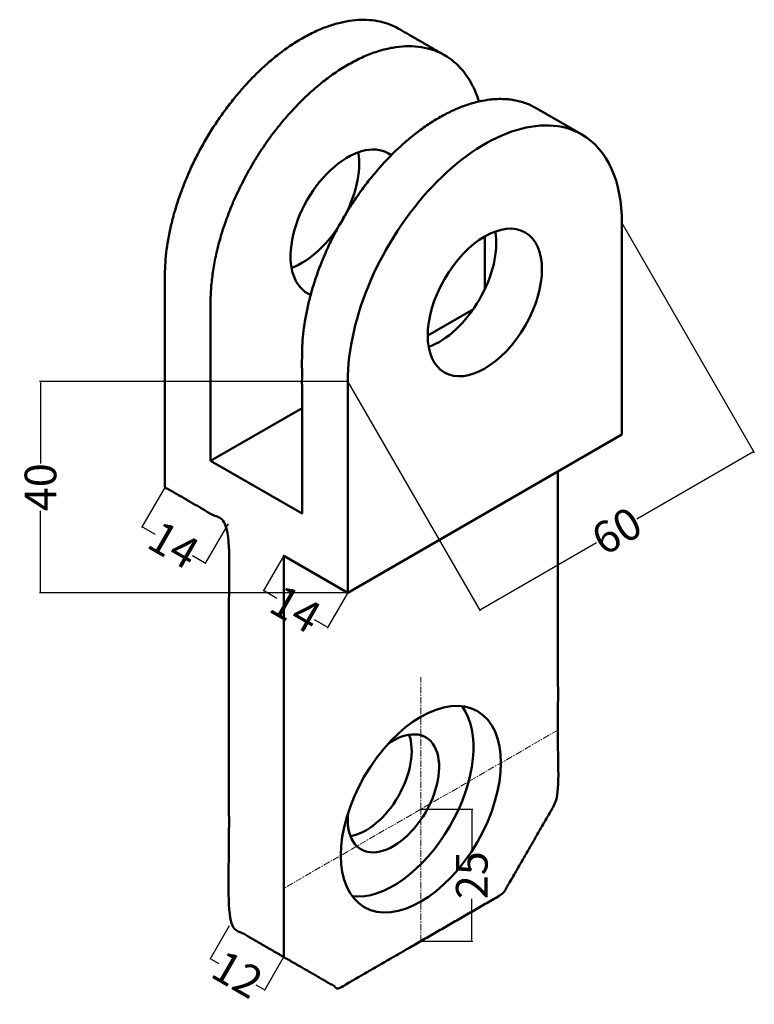
# Model space of a CAD drawing. Units: millimetres. Extents: x 4 to 143, y 22 to 208.
import ezdxf

# ---------------------------------------------------------------- set-up
doc = ezdxf.new("R2010")
doc.units = ezdxf.units.MM
doc.header["$MEASUREMENT"] = 0
doc.linetypes.add('CENTER', pattern=[2, 1.25, -0.25, 0.25, -0.25])
for name, color, linetype, lineweight in [('M-CNTR', 1, 'CENTER', 18), ('M-DIMS', 2, 'Continuous', 25), ('M-OUTL', 7, 'Continuous', 50)]:
    doc.layers.add(name, color=color, linetype=linetype, lineweight=lineweight)
doc.styles.get("Standard").update_dxf_attribs({"font": 'arial.ttf'})
doc.dimstyles.get("Standard").update_dxf_attribs({"dimtxt": 6, "dimasz": 0.18, "dimexe": 0.18, "dimexo": 0.0625, "dimgap": 0.09, "dimtad": 0, "dimtoh": 1, "dimdec": 0, "dimzin": 0, "dimdsep": 46, "dimtxsty": 'Standard', "dimcen": 0.09, "dimadec": 0, "dimazin": 0, "dimtfac": 1, "dimtdec": 0, "dimtofl": 0, "dimtmove": 0, "dimatfit": 3, "dimfxl": 1, "dimtolj": 1, "dimtzin": 0, "dimarcsym": 0})

# ---------------------------------------------------------------- blocks, each defined once
blk = doc.blocks.new('*D1')
at = {"layer": 'Defpoints', "color": 0, "transparency": 16777216}
for p in [(53.96, 106.73), (66.08, 99.73), (62.29, 93.16)]:
    blk.add_point(p, dxfattribs=at)
at = {"layer": 'M-DIMS', "color": 0, "lineweight": -2, "transparency": 16777216}
for p, q in [((53.93, 106.68), (50.07, 100.01)), ((50.32, 100.07), (52.68, 98.71)), ((66.05, 99.68), (62.2, 93.01)), ((62.13, 93.25), (59.77, 94.62))]:
    blk.add_line(p, q, dxfattribs=at)
at = {"layer": 'M-DIMS', "color": 0, "transparency": 16777216}
for points in [[(50.33, 100.1), (50.3, 100.05), (50.16, 100.16)], [(62.15, 93.28), (62.12, 93.23), (62.29, 93.16)]]:
    blk.add_solid(points, dxfattribs=at)
at = {"layer": 'M-DIMS', "color": 0, "transparency": 16777216, "insert": (56.23, 96.66), "char_height": 6, "attachment_point": 5, "rotation": 330}
blk.add_mtext('\\A1;14', dxfattribs=at)
blk = doc.blocks.new('*D2')
at = {"layer": 'Defpoints', "color": 0, "transparency": 16777216}
for p in [(31.44, 119.73), (27.12, 112.26), (43.43, 112.81)]:
    blk.add_point(p, dxfattribs=at)
at = {"layer": 'M-DIMS', "color": 0, "lineweight": -2, "transparency": 16777216}
for p, q in [((31.41, 119.68), (27.03, 112.1)), ((27.28, 112.17), (29.58, 110.84)), ((43.4, 112.76), (39.03, 105.18)), ((38.96, 105.42), (36.67, 106.75))]:
    blk.add_line(p, q, dxfattribs=at)
at = {"layer": 'M-DIMS', "color": 0, "transparency": 16777216}
for points in [[(27.3, 112.19), (27.27, 112.14), (27.12, 112.26)], [(38.98, 105.45), (38.95, 105.4), (39.12, 105.33)]]:
    blk.add_solid(points, dxfattribs=at)
at = {"layer": 'M-DIMS', "color": 0, "transparency": 16777216, "insert": (33.12, 108.79), "char_height": 6, "attachment_point": 5, "rotation": 330}
blk.add_mtext('\\A1;14', dxfattribs=at)
blk = doc.blocks.new('*D3')
at = {"layer": 'Defpoints', "color": 0, "transparency": 16777216}
for p in [(43.66, 36.68), (40.05, 30.42), (53.96, 30.73)]:
    blk.add_point(p, dxfattribs=at)
at = {"layer": 'M-DIMS', "color": 0, "lineweight": -2, "transparency": 16777216}
for p, q in [((43.63, 36.62), (39.96, 30.26)), ((40.21, 30.33), (41.67, 29.49)), ((53.93, 30.68), (50.26, 24.32)), ((50.19, 24.57), (48.73, 25.41))]:
    blk.add_line(p, q, dxfattribs=at)
at = {"layer": 'M-DIMS', "color": 0, "transparency": 16777216}
for points in [[(40.22, 30.36), (40.19, 30.3), (40.05, 30.42)], [(50.2, 24.59), (50.17, 24.54), (50.35, 24.48)]]:
    blk.add_solid(points, dxfattribs=at)
at = {"layer": 'M-DIMS', "color": 0, "transparency": 16777216, "insert": (45.2, 27.45), "char_height": 6, "attachment_point": 5, "rotation": 330}
blk.add_mtext('\\A1;12', dxfattribs=at)
blk = doc.blocks.new('*D4')
at = {"layer": 'Defpoints', "color": 0, "transparency": 16777216}
for p in [(79.94, 58.73), (79.94, 33.73), (89.59, 33.73)]:
    blk.add_point(p, dxfattribs=at)
at = {"layer": 'M-DIMS', "color": 0, "lineweight": -2, "transparency": 16777216}
for p, q in [((80, 58.73), (89.77, 58.73)), ((89.59, 58.55), (89.59, 50.69)), ((89.59, 33.91), (89.59, 41.77)), ((80, 33.73), (89.77, 33.73))]:
    blk.add_line(p, q, dxfattribs=at)
at = {"layer": 'M-DIMS', "color": 0, "transparency": 16777216}
for points in [[(89.56, 58.55), (89.62, 58.55), (89.59, 58.73)], [(89.56, 33.91), (89.62, 33.91), (89.59, 33.73)]]:
    blk.add_solid(points, dxfattribs=at)
at = {"layer": 'M-DIMS', "color": 0, "transparency": 16777216, "insert": (89.59, 46.23), "char_height": 6, "attachment_point": 5, "rotation": 90}
blk.add_mtext('\\A1;25', dxfattribs=at)
blk = doc.blocks.new('*D5')
at = {"layer": 'Defpoints', "color": 0, "transparency": 16777216}
for p in [(118.04, 169.73), (66.08, 139.73), (143.03, 126.46)]:
    blk.add_point(p, dxfattribs=at)
at = {"layer": 'M-DIMS', "color": 0, "lineweight": -2, "transparency": 16777216}
for p, q in [((118.07, 169.68), (143.12, 126.3)), ((66.11, 139.68), (91.16, 96.3)), ((142.87, 126.37), (120.85, 113.65)), ((91.22, 96.55), (113.24, 109.26))]:
    blk.add_line(p, q, dxfattribs=at)
at = {"layer": 'M-DIMS', "color": 0, "transparency": 16777216}
for points in [[(142.86, 126.39), (142.89, 126.34), (143.03, 126.46)], [(91.21, 96.57), (91.24, 96.52), (91.07, 96.46)]]:
    blk.add_solid(points, dxfattribs=at)
at = {"layer": 'M-DIMS', "color": 0, "transparency": 16777216, "insert": (117.05, 111.46), "char_height": 6, "attachment_point": 5, "rotation": 30}
blk.add_mtext('\\A1;60', dxfattribs=at)
blk = doc.blocks.new('*D6')
at = {"layer": 'Defpoints', "color": 0, "transparency": 16777216}
for p in [(66.08, 139.73), (7.87, 99.73), (66.08, 99.73)]:
    blk.add_point(p, dxfattribs=at)
at = {"layer": 'M-DIMS', "color": 0, "lineweight": -2, "transparency": 16777216}
for p, q in [((66.02, 139.73), (7.69, 139.73)), ((7.87, 139.55), (7.87, 124.23)), ((7.87, 99.91), (7.87, 115.24)), ((66.02, 99.73), (7.69, 99.73))]:
    blk.add_line(p, q, dxfattribs=at)
at = {"layer": 'M-DIMS', "color": 0, "transparency": 16777216}
for points in [[(7.84, 139.55), (7.9, 139.55), (7.87, 139.73)], [(7.84, 99.91), (7.9, 99.91), (7.87, 99.73)]]:
    blk.add_solid(points, dxfattribs=at)
at = {"layer": 'M-DIMS', "color": 0, "transparency": 16777216, "insert": (7.87, 119.73), "char_height": 6, "attachment_point": 5, "rotation": 90}
blk.add_mtext('\\A1;40', dxfattribs=at)

msp = doc.modelspace()

# ---------------------------------------------------------------- linework, layer by layer
at = {"layer": 'M-CNTR'}
for points in [[(105.92, 73.73), (79.94, 58.73), (79.94, 83.73)], [(79.94, 33.73), (79.94, 58.73), (53.96, 43.73)]]:
    msp.add_lwpolyline(points, dxfattribs=at)
at = {"layer": 'M-OUTL'}
for p, q in [((110.27, 186.64), (101.77, 191.55)), ((118.04, 129.73), (118.04, 169.73)), ((92.06, 157.23), (92.06, 167.23)), ((81.24, 148.48), (89.9, 153.48)), ((66.08, 139.73), (66.08, 99.73)), ((40.1, 124.73), (57.42, 134.73)), ((66.08, 99.73), (118.04, 129.73)), ((57.42, 114.73), (40.1, 124.73))]:
    msp.add_line(p, q, dxfattribs=at)
msp.add_lwpolyline([(66.08, 99.73), (53.96, 106.73), (53.96, 43.73), (53.96, 30.73)], dxfattribs=at)
for centre, major_axis, start_param, end_param in [((92.06, 154.73), (-18.37, -31.82), 3.141593, 5.497787), ((92.06, 154.73), (-18.37, -31.82), 2.356194, 3.141593), ((66.08, 169.73), (-7.65, -13.26), 3.061959, 6.362819), ((57.42, 174.73), (-7.65, -13.26), 0.601264, 2.540328), ((83.4, 159.73), (-7.65, -13.26), 0.601264, 2.540328), ((74.74, 61.73), (-10.72, -18.56), 0.244877, 2.896716), ((74.74, 61.73), (-6.12, -10.61), 5.37062, 10.337343), ((69.55, 64.73), (-6.12, -10.61), 6.721334, 8.986629)]:
    msp.add_ellipse(centre, major_axis=major_axis, ratio=0.57735, start_param=start_param, end_param=end_param, dxfattribs=at)
for centre, major_axis in [((92.06, 154.73), (-7.65, -13.26)), ((79.94, 58.73), (-10.72, -18.56))]:
    msp.add_ellipse(centre, major_axis=major_axis, ratio=0.57735, dxfattribs=at)
for points, weights, knots in [([(84.45, 201.55), (80.12, 204.05), (75.79, 206.55), (63.52, 213.64), (47.48, 196.71), (31.44, 179.78), (31.44, 159.73), (31.44, 139.73), (31.44, 119.73), (37.5, 116.23), (43.57, 112.73), (43.57, 74.73), (43.57, 36.73), (48.76, 33.73), (53.96, 30.73), (59.15, 27.73), (64.35, 24.73), (79.94, 33.73), (95.53, 42.73), (100.72, 51.73), (105.92, 60.73), (105.92, 91.73), (105.92, 122.73)], [1, 1, 1, 0.831469612303, 1, 0.831469612303, 1, 1, 1, 1, 1, 1, 1, 1, 1, 1, 1, 1, 1, 1, 1, 1, 1], [0, 0, 0, 1, 1, 2.178097, 2.178097, 3.356194, 3.356194, 4.356194, 4.356194, 5.356194, 5.356194, 6.356194, 6.356194, 7.356194, 7.356194, 8.356194, 8.356194, 9.356194, 9.356194, 10.356194, 10.356194, 11.356194, 11.356194, 11.356194]), ([(90.94, 192.8), (84.44, 213.8), (62.27, 197.21), (40.1, 180.61), (40.1, 154.73), (40.1, 139.73), (40.1, 124.73)], [1, 0.757207405252, 1, 0.757207405252, 1, 1, 1], [0, 0, 0, 1.423539, 1.423539, 2.847077, 2.847077, 3.847077, 3.847077, 3.847077]), ([(101.78, 191.55), (89.5, 198.64), (73.46, 181.71), (57.42, 164.78), (57.42, 144.73), (57.42, 129.73), (57.42, 114.73)], [1, 0.831447260419, 1, 0.831447260419, 1, 1, 1], [0, 0, 0, 1.178178, 1.178178, 2.356355, 2.356355, 3.356355, 3.356355, 3.356355]), ([(74.4, 166.54), (73.77, 165.3), (73.01, 164.12), (73.77, 165.3), (74.4, 166.54)], [1, 0.995842050171, 1, 0.995842050171, 1], [0, 0, 0, 0.1824464, 0.1824464, 0.3648927, 0.3648927, 0.3648927])]:
    msp.add_rational_spline(points, weights, degree=2, knots=knots, dxfattribs=at)

# ---------------------------------------------------------------- dimensions: what is measured, and where the dimension line sits
at = {"layer": 'M-DIMS'}
for p1, p2, distance, picture, middle in [((66.08, 139.73), (118.04, 169.73), -49.97, '*D5', (117.05, 111.46)), ((66.08, 139.73), (66.08, 99.73), -58.21, '*D6', (7.87, 119.73)), ((43.43, 112.81), (31.44, 119.73), 8.63, '*D2', (33.12, 108.79)), ((53.96, 106.73), (66.08, 99.73), -7.59, '*D1', (56.23, 96.66)), ((79.94, 58.73), (79.94, 33.73), 9.65, '*D4', (89.59, 46.23)), ((53.96, 30.73), (43.66, 36.68), 7.22, '*D3', (45.2, 27.45))]:
    dim = msp.add_aligned_dim(p1=p1, p2=p2, distance=distance, dimstyle='Standard', override={"dimclrd": 0, "dimclre": 0, "dimclrt": 0}, dxfattribs=at)
    dim.commit()
    dim.dimension.update_dxf_attribs({"geometry": picture, "text_midpoint": middle})

doc.saveas('drawing.dxf')
